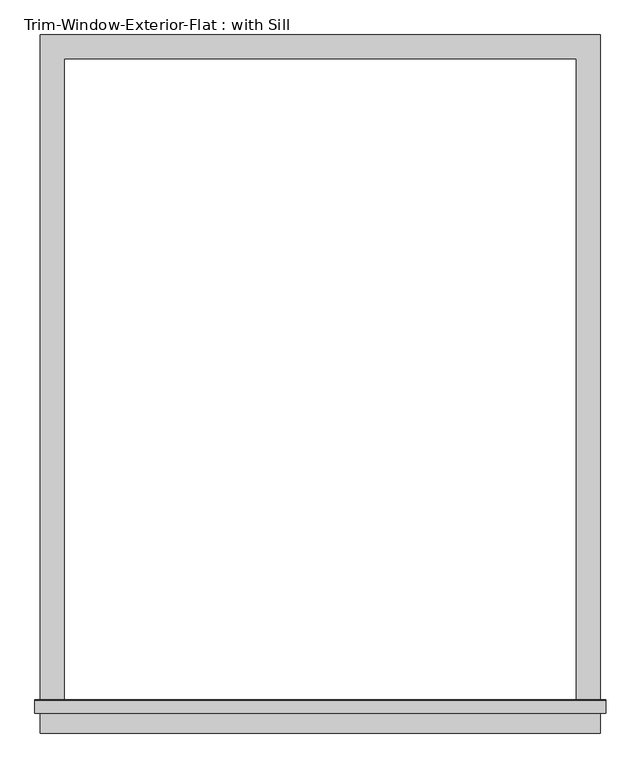
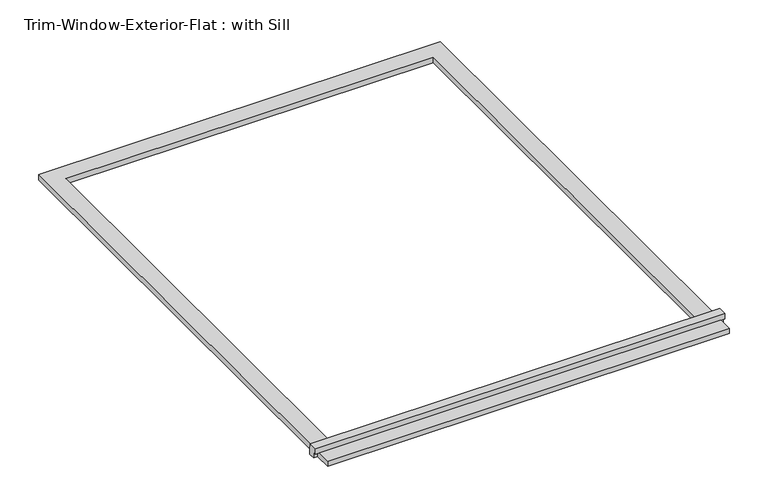
"""IFC4 building model written with IfcOpenShell, lengths in millimetres: proxy geometry, Trim-Window-Exterior-Flat : with Sill."""

from ifc_helpers import new_model, si_unit, frame, origin, origin_with_axes, place, context, project, spatial, polyline, outline, extrude, source, transform, mapped, element, save


def trim_window_exterior_flat_with_sill_92b9b949(model_context):
    return source(origin(), model_context, "Body", "SweptSolid", [
        extrude(outline(polyline([(666.75, -1546.1823709), (666.75, -1603.3323709), (-666.75, -1603.3323709), (-666.75, -1546.1823709), (666.75, -1546.1823709)])), origin_with_axes(), (0.0, 0.0, 1.0), 19.05),
        extrude(outline(polyline([(-1555.75, 38.1), (-1526.4580645, 38.1), (-1524.0, 19.05), (-1524.0, 0.0), (-1546.1823709, 0.0), (-1546.1823709, 19.05), (-1555.75, 19.05), (-1555.75, 38.1)])), frame((-679.45, 0.0, 0.0), z_axis=(1.0, 0.0, 0.0), x_axis=(0.0, 1.0, 0.0)), (0.0, 0.0, 1.0), 1358.9),
        extrude(outline(polyline([(-666.75, 57.15), (666.75, 57.15), (666.75, -1524.0), (609.6, -1524.0), (609.6, 0.0), (-609.6, 0.0), (-609.6, -1524.0), (-666.75, -1524.0), (-666.75, 57.15)])), origin_with_axes(), (0.0, 0.0, 1.0), 19.05),
    ])


if __name__ == "__main__":
    model = new_model("IFC4")
    model_context = context("Model", 3, world=origin())
    ifc_project = project(units=[si_unit("LENGTHUNIT", "METRE", prefix="MILLI")], contexts=[model_context])
    site = spatial("IfcSite", under=ifc_project)
    building = spatial("IfcBuilding", under=site)
    placement = place(None, origin())
    trim_window_exterior_flat_with_sill_shape = trim_window_exterior_flat_with_sill_92b9b949(model_context)
    element("IfcBuildingElementProxy", 1, Name="Trim-Window-Exterior-Flat : with Sill", ObjectType="Trim-Window-Exterior-Flat : with Sill", at=placement, inside=building, context=model_context, shape_type="MappedRepresentation", body=[
        mapped(trim_window_exterior_flat_with_sill_shape, transform((0.0, 0.0, 0.0), x_axis=(1.0, 0.0, 0.0), y_axis=(0.0, 1.0, 0.0), z_axis=(0.0, 0.0, 1.0))),
    ])
    save(model, "model.ifc")

# Revit data of these elements
# Type "Trim-Window-Exterior-Flat : with Sill"
#   Trim Width = 0' - 2 1/4"
#   Trim Thickness_Picture Frame = 0' - 1 1/4"
#   Trim Thickness_with Sill = 0' - 0 3/4"
#   Sill Thickness = 0' - 1 1/4"
#   Opening Width [instance default] = 2' - 0"
#   Opening Height [instance default] = 3' - 0"
#   Default Elevation = 4' - 0"
#   Sill = yes
#   Picture Frame = no
#   Trim Material [instance default] = none
# Element 1 (IfcBuildingElementProxy, "Trim-Window-Exterior-Flat : with Sill")
#   Opening Width = 4' - 0"
#   Opening Height = 5' - 0"
#   Trim Material = BLACK MATERIAL
#   Materials on its faces: "BLACK MATERIAL"
# Materials
#   "BLACK MATERIAL": class "Generic", colour RGB 120 120 120, transparency 0, Cost = 0
